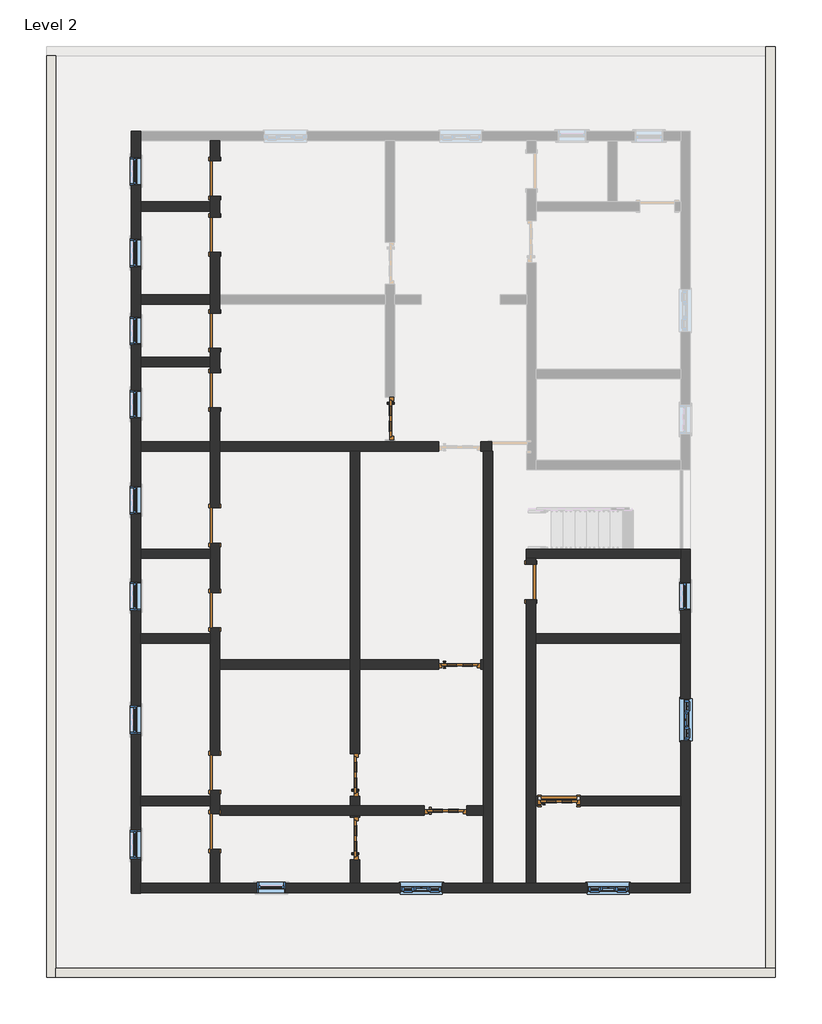
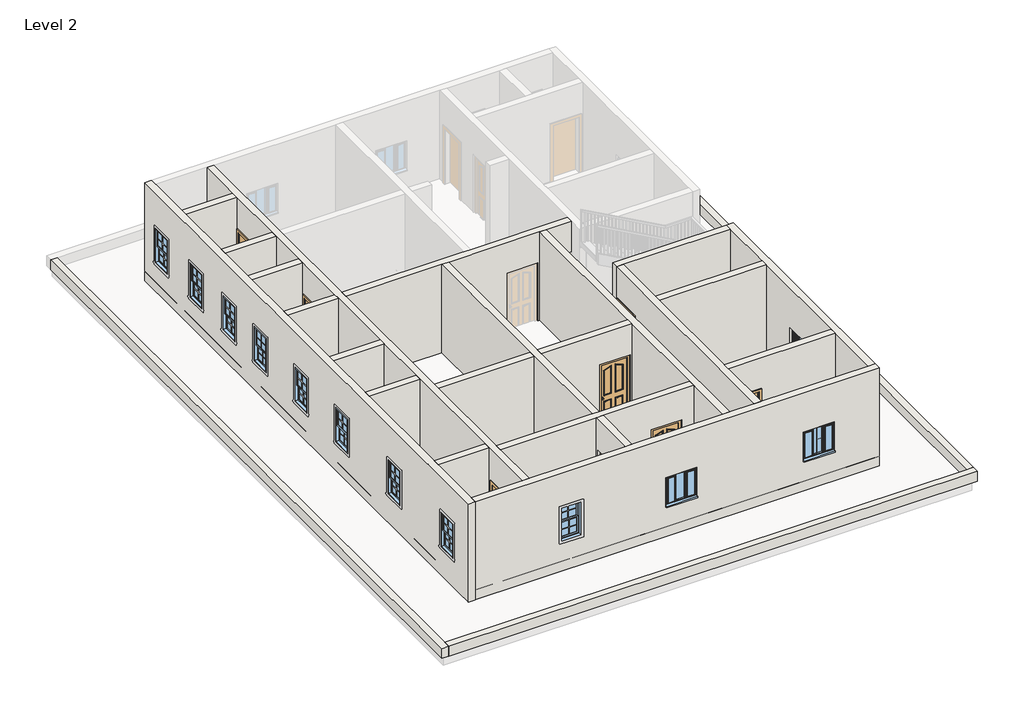
# One storey, part 1 of 3: 22 walls, 16 doors, 13 windows.
"""IFC4 building model written with IfcOpenShell, lengths in millimetres."""

from ifc_helpers import new_model, si_unit, frame, origin, place, context, project, spatial, polyline, outline, extrude, faceted_brep, transform, mapped, element, save
from components import doors_extsgl_12_910x2110mm_9a09825e, doors_extsgl_12_910x2110mm_ece77ece, door_fadea3f2, door_53b1b562, window_679d2811, windows_tpl_w_glazing_cross_bars_910x910mm_4aa0f884

model = new_model("IFC4")

# Units and contexts
model_context = context("Model", 3, world=origin())
ifc_project = project(units=[si_unit("LENGTHUNIT", "METRE", prefix="MILLI")], contexts=[model_context])

# Site, building, storey
site = spatial("IfcSite", under=ifc_project)
building = spatial("IfcBuilding", under=site)
storey = spatial("IfcBuildingStorey", under=building, Name="Level 2", Elevation=3048.0)

# Doors
placement = place(None, origin())
doors_extsgl_12_910x2110mm_shape = doors_extsgl_12_910x2110mm_9a09825e(model_context)
element("IfcDoor", 1, ObjectType="Doors_ExtSgl_12 : 910x2110mm", at=placement, inside=storey, context=model_context, shape_type="MappedRepresentation", body=[
    mapped(doors_extsgl_12_910x2110mm_shape, transform((-4887.6876145, 1213.3404944, 3048.0), x_axis=(0.0, -1.0, 0.0), y_axis=(1.0, 0.0, 0.0), z_axis=(0.0, 0.0, 1.0))),
])
doors_extsgl_12_910x2110mm_2_shape = doors_extsgl_12_910x2110mm_ece77ece(model_context)
element("IfcDoor", 2, ObjectType="Doors_ExtSgl_12 : 910x2110mm", at=placement, inside=storey, context=model_context, shape_type="MappedRepresentation", body=[
    mapped(doors_extsgl_12_910x2110mm_2_shape, transform((-5649.6876145, -6482.8595056, 3048.0), x_axis=(0.0, 1.0, 0.0), y_axis=(-1.0, 0.0, 0.0), z_axis=(0.0, 0.0, 1.0))),
])
element("IfcDoor", 3, ObjectType="Doors_ExtSgl_12 : 910x2110mm", at=placement, inside=storey, context=model_context, shape_type="MappedRepresentation", body=[
    mapped(doors_extsgl_12_910x2110mm_2_shape, transform((-1242.7876145, -7041.6595056, 3048.0), x_axis=(1.0, 0.0, 0.0), y_axis=(0.0, 1.0, 0.0), z_axis=(0.0, 0.0, 1.0))),
])
element("IfcDoor", 4, ObjectType="Doors_ExtSgl_12 : 910x2110mm", at=placement, inside=storey, context=model_context, shape_type="MappedRepresentation", body=[
    mapped(doors_extsgl_12_910x2110mm_2_shape, transform((-5649.6876145, -7854.4595056, 3048.0), x_axis=(0.0, 1.0, 0.0), y_axis=(-1.0, 0.0, 0.0), z_axis=(0.0, 0.0, 1.0))),
])
element("IfcDoor", 5, ObjectType="Doors_ExtSgl_12 : 910x2110mm", at=placement, inside=storey, context=model_context, shape_type="MappedRepresentation", body=[
    mapped(doors_extsgl_12_910x2110mm_2_shape, transform((-3693.8876145, -7244.8595056, 3048.0), x_axis=(1.0, 0.0, 0.0), y_axis=(0.0, 1.0, 0.0), z_axis=(0.0, 0.0, 1.0))),
])
element("IfcDoor", 6, ObjectType="Doors_ExtSgl_12 : 910x2110mm", at=placement, inside=storey, context=model_context, shape_type="MappedRepresentation", body=[
    mapped(doors_extsgl_12_910x2110mm_2_shape, transform((-3389.0876145, -4095.2595056, 3048.0), x_axis=(1.0, 0.0, 0.0), y_axis=(0.0, 1.0, 0.0), z_axis=(0.0, 0.0, 1.0))),
])
door_shape = door_fadea3f2(model_context)
element("IfcDoor", 7, ObjectType="Single-Flush : 30\" x 80\"", at=placement, inside=storey, context=model_context, shape_type="MappedRepresentation", body=[
    mapped(door_shape, transform((-8672.2876145, 5175.7404944, 3048.0), x_axis=(0.0, 1.0, 0.0), y_axis=(-1.0, 0.0, 0.0), z_axis=(0.0, 0.0, 1.0))),
])
element("IfcDoor", 8, ObjectType="Single-Flush : 30\" x 80\"", at=placement, inside=storey, context=model_context, shape_type="MappedRepresentation", body=[
    mapped(door_shape, transform((-8672.2876145, -7702.0595056, 3048.0), x_axis=(0.0, 1.0, 0.0), y_axis=(-1.0, 0.0, 0.0), z_axis=(0.0, 0.0, 1.0))),
])
element("IfcDoor", 9, ObjectType="Single-Flush : 30\" x 80\"", at=placement, inside=storey, context=model_context, shape_type="MappedRepresentation", body=[
    mapped(door_shape, transform((-1852.3876145, -2317.2595056, 3048.0), x_axis=(0.0, -1.0, 0.0), y_axis=(1.0, 0.0, 0.0), z_axis=(0.0, 0.0, 1.0))),
])
element("IfcDoor", 10, ObjectType="Single-Flush : 30\" x 80\"", at=placement, inside=storey, context=model_context, shape_type="MappedRepresentation", body=[
    mapped(door_shape, transform((-1242.7876145, -7041.6595056, 3048.0), x_axis=(1.0, 0.0, 0.0), y_axis=(0.0, 1.0, 0.0), z_axis=(0.0, 0.0, 1.0))),
])
door_2_shape = door_53b1b562(model_context)
element("IfcDoor", 11, ObjectType="Single-Flush : 30\" x 80\"", at=placement, inside=storey, context=model_context, shape_type="MappedRepresentation", body=[
    mapped(door_2_shape, transform((-8672.2876145, 6394.9404944, 3048.0), x_axis=(0.0, -1.0, 0.0), y_axis=(1.0, 0.0, 0.0), z_axis=(0.0, 0.0, 1.0))),
])
element("IfcDoor", 12, ObjectType="Single-Flush : 30\" x 80\"", at=placement, inside=storey, context=model_context, shape_type="MappedRepresentation", body=[
    mapped(door_2_shape, transform((-8672.2876145, 3105.6404944, 3048.0), x_axis=(0.0, -1.0, 0.0), y_axis=(1.0, 0.0, 0.0), z_axis=(0.0, 0.0, 1.0))),
])
element("IfcDoor", 13, ObjectType="Single-Flush : 30\" x 80\"", at=placement, inside=storey, context=model_context, shape_type="MappedRepresentation", body=[
    mapped(door_2_shape, transform((-8672.2876145, 1822.9404944, 3048.0), x_axis=(0.0, -1.0, 0.0), y_axis=(1.0, 0.0, 0.0), z_axis=(0.0, 0.0, 1.0))),
])
element("IfcDoor", 14, ObjectType="Single-Flush : 30\" x 80\"", at=placement, inside=storey, context=model_context, shape_type="MappedRepresentation", body=[
    mapped(door_2_shape, transform((-8672.2876145, -1098.0595056, 3048.0), x_axis=(0.0, -1.0, 0.0), y_axis=(1.0, 0.0, 0.0), z_axis=(0.0, 0.0, 1.0))),
])
element("IfcDoor", 15, ObjectType="Single-Flush : 30\" x 80\"", at=placement, inside=storey, context=model_context, shape_type="MappedRepresentation", body=[
    mapped(door_2_shape, transform((-8672.2876145, -2926.8595056, 3048.0), x_axis=(0.0, -1.0, 0.0), y_axis=(1.0, 0.0, 0.0), z_axis=(0.0, 0.0, 1.0))),
])
element("IfcDoor", 16, ObjectType="Single-Flush : 30\" x 80\"", at=placement, inside=storey, context=model_context, shape_type="MappedRepresentation", body=[
    mapped(door_2_shape, transform((-8672.2876145, -6432.0595056, 3048.0), x_axis=(0.0, -1.0, 0.0), y_axis=(1.0, 0.0, 0.0), z_axis=(0.0, 0.0, 1.0))),
])

# Walls
element("IfcWall", 17, ObjectType="4.5\"", at=placement, inside=storey, context=model_context, shape_type="Brep", body=[
    faceted_brep([(-8773.8876145, -6813.0595056, 3048.0), (-8773.8876145, -6940.0595056, 3048.0), (-8773.8876145, -7143.2595056, 3048.0), (-8773.8876145, -7321.0595056, 3048.0), (-8773.8876145, -7321.0595056, 5080.0), (-8773.8876145, -8083.0595056, 5080.0), (-8773.8876145, -8083.0595056, 3048.0), (-8773.8876145, -8819.6595056, 3048.0), (-8773.8876145, -8819.6595056, 6096.0), (-8773.8876145, -7143.2595056, 6096.0), (-8773.8876145, -6940.0595056, 6096.0), (-8773.8876145, -3638.0595056, 6096.0), (-8773.8876145, -3434.8595056, 6096.0), (-8773.8876145, -1809.2595056, 6096.0), (-8773.8876145, -1606.0595056, 6096.0), (-8773.8876145, 502.1404944, 6096.0), (-8773.8876145, 705.3404944, 6096.0), (-8773.8876145, 2330.9404944, 6096.0), (-8773.8876145, 2534.1404944, 6096.0), (-8773.8876145, 3677.1404944, 6096.0), (-8773.8876145, 3880.3404944, 6096.0), (-8773.8876145, 5683.7404944, 6096.0), (-8773.8876145, 5886.9404944, 6096.0), (-8773.8876145, 7207.7404944, 6096.0), (-8773.8876145, 7207.7404944, 3048.0), (-8773.8876145, 6775.9404944, 3048.0), (-8773.8876145, 6775.9404944, 5080.0), (-8773.8876145, 6013.9404944, 5080.0), (-8773.8876145, 6013.9404944, 3048.0), (-8773.8876145, 5886.9404944, 3048.0), (-8773.8876145, 5683.7404944, 3048.0), (-8773.8876145, 5556.7404944, 3048.0), (-8773.8876145, 5556.7404944, 5080.0), (-8773.8876145, 4794.7404944, 5080.0), (-8773.8876145, 4794.7404944, 3048.0), (-8773.8876145, 3880.3404944, 3048.0), (-8773.8876145, 3677.1404944, 3048.0), (-8773.8876145, 3486.6404944, 3048.0), (-8773.8876145, 3486.6404944, 5080.0), (-8773.8876145, 2724.6404944, 5080.0), (-8773.8876145, 2724.6404944, 3048.0), (-8773.8876145, 2534.1404944, 3048.0), (-8773.8876145, 2330.9404944, 3048.0), (-8773.8876145, 2203.9404944, 3048.0), (-8773.8876145, 2203.9404944, 5080.0), (-8773.8876145, 1441.9404944, 5080.0), (-8773.8876145, 1441.9404944, 3048.0), (-8773.8876145, 705.3404944, 3048.0), (-8773.8876145, 502.1404944, 3048.0), (-8773.8876145, -717.0595056, 3048.0), (-8773.8876145, -717.0595056, 5080.0), (-8773.8876145, -1479.0595056, 5080.0), (-8773.8876145, -1479.0595056, 3048.0), (-8773.8876145, -1606.0595056, 3048.0), (-8773.8876145, -1809.2595056, 3048.0), (-8773.8876145, -2545.8595056, 3048.0), (-8773.8876145, -2545.8595056, 5080.0), (-8773.8876145, -3307.8595056, 5080.0), (-8773.8876145, -3307.8595056, 3048.0), (-8773.8876145, -3434.8595056, 3048.0), (-8773.8876145, -3638.0595056, 3048.0), (-8773.8876145, -6051.0595056, 3048.0), (-8773.8876145, -6051.0595056, 5080.0), (-8773.8876145, -6813.0595056, 5080.0), (-8570.6876145, -7321.0595056, 5080.0), (-8570.6876145, -7321.0595056, 3048.0), (-8570.6876145, -7143.2595056, 3048.0), (-8570.6876145, -6813.0595056, 3048.0), (-8570.6876145, -6813.0595056, 5080.0), (-8570.6876145, -6051.0595056, 5080.0), (-8570.6876145, -6051.0595056, 3048.0), (-8570.6876145, -4196.8595056, 3048.0), (-8570.6876145, -3993.6595056, 3048.0), (-8570.6876145, -3307.8595056, 3048.0), (-8570.6876145, -3307.8595056, 5080.0), (-8570.6876145, -2545.8595056, 5080.0), (-8570.6876145, -2545.8595056, 3048.0), (-8570.6876145, -1479.0595056, 3048.0), (-8570.6876145, -1479.0595056, 5080.0), (-8570.6876145, -717.0595056, 5080.0), (-8570.6876145, -717.0595056, 3048.0), (-8570.6876145, 502.1404944, 3048.0), (-8570.6876145, 705.3404944, 3048.0), (-8570.6876145, 1441.9404944, 3048.0), (-8570.6876145, 1441.9404944, 5080.0), (-8570.6876145, 2203.9404944, 5080.0), (-8570.6876145, 2203.9404944, 3048.0), (-8570.6876145, 2724.6404944, 3048.0), (-8570.6876145, 2724.6404944, 5080.0), (-8570.6876145, 3486.6404944, 5080.0), (-8570.6876145, 3486.6404944, 3048.0), (-8570.6876145, 3677.1404944, 3048.0), (-8570.6876145, 3880.3404944, 3048.0), (-8570.6876145, 4794.7404944, 3048.0), (-8570.6876145, 4794.7404944, 5080.0), (-8570.6876145, 5556.7404944, 5080.0), (-8570.6876145, 5556.7404944, 3048.0), (-8570.6876145, 6013.9404944, 3048.0), (-8570.6876145, 6013.9404944, 5080.0), (-8570.6876145, 6775.9404944, 5080.0), (-8570.6876145, 6775.9404944, 3048.0), (-8570.6876145, 7207.7404944, 3048.0), (-8570.6876145, 7207.7404944, 6096.0), (-8570.6876145, 3880.3404944, 6096.0), (-8570.6876145, 3677.1404944, 6096.0), (-8570.6876145, 705.3404944, 6096.0), (-8570.6876145, 502.1404944, 6096.0), (-8570.6876145, -3993.6595056, 6096.0), (-8570.6876145, -4196.8595056, 6096.0), (-8570.6876145, -7143.2595056, 6096.0), (-8570.6876145, -7346.4595056, 6096.0), (-8570.6876145, -8819.6595056, 6096.0), (-8570.6876145, -8819.6595056, 3048.0), (-8570.6876145, -8083.0595056, 3048.0), (-8570.6876145, -8083.0595056, 5080.0)], [[[0, 1, 2, 3, 4, 5, 6, 7, 8, 9, 10, 11, 12, 13, 14, 15, 16, 17, 18, 19, 20, 21, 22, 23, 24, 25, 26, 27, 28, 29, 30, 31, 32, 33, 34, 35, 36, 37, 38, 39, 40, 41, 42, 43, 44, 45, 46, 47, 48, 49, 50, 51, 52, 53, 54, 55, 56, 57, 58, 59, 60, 61, 62, 63]], [[64, 65, 66, 67, 68, 69, 70, 71, 72, 73, 74, 75, 76, 77, 78, 79, 80, 81, 82, 83, 84, 85, 86, 87, 88, 89, 90, 91, 92, 93, 94, 95, 96, 97, 98, 99, 100, 101, 102, 103, 104, 105, 106, 107, 108, 109, 110, 111, 112, 113, 114]], [[25, 24, 101, 100]], [[97, 96, 31, 30, 29, 28]], [[37, 36, 35, 34, 93, 92, 91, 90]], [[43, 42, 41, 40, 87, 86]], [[49, 48, 47, 46, 83, 82, 81, 80]], [[55, 54, 53, 52, 77, 76]], [[61, 60, 59, 58, 73, 72, 71, 70]], [[113, 112, 7, 6]], [[67, 66, 65, 3, 2, 1, 0]], [[23, 22, 21, 20, 19, 18, 17, 16, 15, 14, 13, 12, 11, 10, 9, 8, 111, 110, 109, 108, 107, 106, 105, 104, 103, 102]], [[8, 7, 112, 111]], [[24, 23, 102, 101]], [[98, 97, 28, 27]], [[99, 98, 27, 26]], [[100, 99, 26, 25]], [[32, 31, 96, 95]], [[33, 32, 95, 94]], [[34, 33, 94, 93]], [[88, 87, 40, 39]], [[89, 88, 39, 38]], [[90, 89, 38, 37]], [[84, 83, 46, 45]], [[85, 84, 45, 44]], [[86, 85, 44, 43]], [[78, 77, 52, 51]], [[79, 78, 51, 50]], [[80, 79, 50, 49]], [[74, 73, 58, 57]], [[75, 74, 57, 56]], [[76, 75, 56, 55]], [[68, 67, 0, 63]], [[69, 68, 63, 62]], [[70, 69, 62, 61]], [[4, 3, 65, 64]], [[5, 4, 64, 114]], [[6, 5, 114, 113]]]),
])
element("IfcWall", 18, ObjectType="4.5\"", at=placement, inside=storey, context=model_context, shape_type="SweptSolid", body=[
    extrude(outline(polyline([(-8773.8876145, 5683.7404944), (-10272.4876145, 5683.7404944), (-10272.4876145, 5886.9404944), (-8773.8876145, 5886.9404944), (-8773.8876145, 5683.7404944)])), frame((0.0, 0.0, 3048.0), z_axis=(0.0, 0.0, 1.0), x_axis=(1.0, 0.0, 0.0)), (0.0, 0.0, 1.0), 3048.0),
])
element("IfcWall", 19, ObjectType="4.5\"", at=placement, inside=storey, context=model_context, shape_type="SweptSolid", body=[
    extrude(outline(polyline([(-8773.8876145, 3677.1404944), (-10272.4876145, 3677.1404944), (-10272.4876145, 3880.3404944), (-8773.8876145, 3880.3404944), (-8773.8876145, 3677.1404944)])), frame((0.0, 0.0, 3048.0), z_axis=(0.0, 0.0, 1.0), x_axis=(1.0, 0.0, 0.0)), (0.0, 0.0, 1.0), 3048.0),
])
element("IfcWall", 20, ObjectType="4.5\"", at=placement, inside=storey, context=model_context, shape_type="SweptSolid", body=[
    extrude(outline(polyline([(-8773.8876145, 2330.9404944), (-10272.4876145, 2330.9404944), (-10272.4876145, 2534.1404944), (-8773.8876145, 2534.1404944), (-8773.8876145, 2330.9404944)])), frame((0.0, 0.0, 3048.0), z_axis=(0.0, 0.0, 1.0), x_axis=(1.0, 0.0, 0.0)), (0.0, 0.0, 1.0), 3048.0),
])
element("IfcWall", 21, ObjectType="4.5\"", at=placement, inside=storey, context=model_context, shape_type="Brep", body=[
    faceted_brep([(-10272.4876145, 502.1404944, 6096.0), (-10272.4876145, 502.1404944, 3048.0), (-8773.8876145, 502.1404944, 3048.0), (-8773.8876145, 502.1404944, 6096.0), (-10272.4876145, 705.3404944, 3048.0), (-10272.4876145, 705.3404944, 6096.0), (-8773.8876145, 705.3404944, 6096.0), (-8773.8876145, 705.3404944, 3048.0)], [[[0, 1, 2, 3]], [[4, 5, 6, 7]], [[1, 4, 7, 2]], [[5, 0, 3, 6]], [[1, 0, 5, 4]], [[3, 2, 7, 6]]]),
    faceted_brep([(-1941.2876145, 502.1404944, 5080.0), (-1941.2876145, 502.1404944, 6096.0), (-2677.8876145, 502.1404944, 6096.0), (-2881.0876145, 502.1404944, 6096.0), (-5548.0876145, 502.1404944, 6096.0), (-5751.2876145, 502.1404944, 6096.0), (-8570.6876145, 502.1404944, 6096.0), (-8570.6876145, 502.1404944, 3048.0), (-5751.2876145, 502.1404944, 3048.0), (-5548.0876145, 502.1404944, 3048.0), (-3844.0876145, 502.1404944, 3048.0), (-3844.0876145, 502.1404944, 5158.0), (-2934.0876145, 502.1404944, 5158.0), (-2934.0876145, 502.1404944, 3048.0), (-2881.0876145, 502.1404944, 3048.0), (-2690.5876145, 502.1404944, 3048.0), (-2690.5876145, 502.1404944, 5080.0), (-1941.2876145, 705.3404944, 6096.0), (-1941.2876145, 705.3404944, 5080.0), (-2690.5876145, 705.3404944, 5080.0), (-2690.5876145, 705.3404944, 3048.0), (-2934.0876145, 705.3404944, 3048.0), (-2934.0876145, 705.3404944, 5158.0), (-3844.0876145, 705.3404944, 5158.0), (-3844.0876145, 705.3404944, 3048.0), (-4786.0876145, 705.3404944, 3048.0), (-4989.2876145, 705.3404944, 3048.0), (-8570.6876145, 705.3404944, 3048.0), (-8570.6876145, 705.3404944, 6096.0), (-4989.2876145, 705.3404944, 6096.0), (-4786.0876145, 705.3404944, 6096.0)], [[[0, 1, 2, 3, 4, 5, 6, 7, 8, 9, 10, 11, 12, 13, 14, 15, 16]], [[17, 18, 19, 20, 21, 22, 23, 24, 25, 26, 27, 28, 29, 30]], [[20, 15, 14, 13, 21]], [[24, 10, 9, 8, 7, 27, 26, 25]], [[1, 17, 30, 29, 28, 6, 5, 4, 3, 2]], [[7, 6, 28, 27]], [[17, 1, 0, 18]], [[16, 19, 18, 0]], [[19, 16, 15, 20]], [[24, 23, 11, 10]], [[22, 21, 13, 12]], [[23, 22, 12, 11]]]),
])
element("IfcWall", 22, ObjectType="4.5\"", at=placement, inside=storey, context=model_context, shape_type="SweptSolid", body=[
    extrude(outline(polyline([(-8773.8876145, -1809.2595056), (-10272.4876145, -1809.2595056), (-10272.4876145, -1606.0595056), (-8773.8876145, -1606.0595056), (-8773.8876145, -1809.2595056)])), frame((0.0, 0.0, 3048.0), z_axis=(0.0, 0.0, 1.0), x_axis=(1.0, 0.0, 0.0)), (0.0, 0.0, 1.0), 3048.0),
])
element("IfcWall", 23, ObjectType="4.5\"", at=placement, inside=storey, context=model_context, shape_type="SweptSolid", body=[
    extrude(outline(polyline([(-8773.8876145, -3638.0595056), (-10272.4876145, -3638.0595056), (-10272.4876145, -3434.8595056), (-8773.8876145, -3434.8595056), (-8773.8876145, -3638.0595056)])), frame((0.0, 0.0, 3048.0), z_axis=(0.0, 0.0, 1.0), x_axis=(1.0, 0.0, 0.0)), (0.0, 0.0, 1.0), 3048.0),
])
element("IfcWall", 24, ObjectType="4.5\"", at=placement, inside=storey, context=model_context, shape_type="SweptSolid", body=[
    extrude(outline(polyline([(-8773.8876145, -7143.2595056), (-10272.4876145, -7143.2595056), (-10272.4876145, -6940.0595056), (-8773.8876145, -6940.0595056), (-8773.8876145, -7143.2595056)])), frame((0.0, 0.0, 3048.0), z_axis=(0.0, 0.0, 1.0), x_axis=(1.0, 0.0, 0.0)), (0.0, 0.0, 1.0), 3048.0),
])
element("IfcWall", 25, ObjectType="4.5\"", at=placement, inside=storey, context=model_context, shape_type="Brep", body=[
    faceted_brep([(-3238.8876145, -7346.4595056, 5158.0), (-3238.8876145, -7346.4595056, 3048.0), (-2881.0876145, -7346.4595056, 3048.0), (-2881.0876145, -7346.4595056, 6096.0), (-5548.0876145, -7346.4595056, 6096.0), (-5751.2876145, -7346.4595056, 6096.0), (-8570.6876145, -7346.4595056, 6096.0), (-8570.6876145, -7346.4595056, 3048.0), (-5751.2876145, -7346.4595056, 3048.0), (-5548.0876145, -7346.4595056, 3048.0), (-4148.8876145, -7346.4595056, 3048.0), (-4148.8876145, -7346.4595056, 5158.0), (-2881.0876145, -7143.2595056, 3048.0), (-3238.8876145, -7143.2595056, 3048.0), (-3238.8876145, -7143.2595056, 5158.0), (-4148.8876145, -7143.2595056, 5158.0), (-4148.8876145, -7143.2595056, 3048.0), (-5548.0876145, -7143.2595056, 3048.0), (-5751.2876145, -7143.2595056, 3048.0), (-8570.6876145, -7143.2595056, 3048.0), (-8570.6876145, -7143.2595056, 6096.0), (-5751.2876145, -7143.2595056, 6096.0), (-5548.0876145, -7143.2595056, 6096.0), (-2881.0876145, -7143.2595056, 6096.0), (-8570.6876145, -7321.0595056, 3048.0)], [[[0, 1, 2, 3, 4, 5, 6, 7, 8, 9, 10, 11]], [[12, 13, 14, 15, 16, 17, 18, 19, 20, 21, 22, 23]], [[2, 1, 13, 12]], [[10, 9, 8, 7, 24, 19, 18, 17, 16]], [[6, 5, 4, 3, 23, 22, 21, 20]], [[7, 6, 20, 19, 24]], [[3, 2, 12, 23]], [[16, 15, 11, 10]], [[14, 13, 1, 0]], [[15, 14, 0, 11]]]),
])
element("IfcWall", 26, ObjectType="4.5\"", at=placement, inside=storey, context=model_context, shape_type="Brep", body=[
    faceted_brep([(-5751.2876145, -8819.6595056, 3048.0), (-5751.2876145, -8819.6595056, 6096.0), (-5751.2876145, -7346.4595056, 6096.0), (-5751.2876145, -7346.4595056, 3048.0), (-5751.2876145, -7399.4595056, 3048.0), (-5751.2876145, -7399.4595056, 5158.0), (-5751.2876145, -8309.4595056, 5158.0), (-5751.2876145, -8309.4595056, 3048.0), (-5548.0876145, -8819.6595056, 6096.0), (-5548.0876145, -8819.6595056, 3048.0), (-5548.0876145, -8309.4595056, 3048.0), (-5548.0876145, -8309.4595056, 5158.0), (-5548.0876145, -7399.4595056, 5158.0), (-5548.0876145, -7399.4595056, 3048.0), (-5548.0876145, -7346.4595056, 3048.0), (-5548.0876145, -7346.4595056, 6096.0)], [[[0, 1, 2, 3, 4, 5, 6, 7]], [[8, 9, 10, 11, 12, 13, 14, 15]], [[9, 0, 7, 10]], [[13, 4, 3, 14]], [[1, 8, 15, 2]], [[1, 0, 9, 8]], [[3, 2, 15, 14]], [[7, 6, 11, 10]], [[5, 4, 13, 12]], [[6, 5, 12, 11]]]),
    faceted_brep([(-5751.2876145, 502.1404944, 6096.0), (-5751.2876145, 502.1404944, 3048.0), (-5751.2876145, -3993.6595056, 3048.0), (-5751.2876145, -4196.8595056, 3048.0), (-5751.2876145, -6027.8595056, 3048.0), (-5751.2876145, -6027.8595056, 5158.0), (-5751.2876145, -6937.8595056, 5158.0), (-5751.2876145, -6937.8595056, 3048.0), (-5751.2876145, -7143.2595056, 3048.0), (-5751.2876145, -7143.2595056, 6096.0), (-5751.2876145, -4196.8595056, 6096.0), (-5751.2876145, -3993.6595056, 6096.0), (-5548.0876145, 502.1404944, 3048.0), (-5548.0876145, 502.1404944, 6096.0), (-5548.0876145, -3993.6595056, 6096.0), (-5548.0876145, -4196.8595056, 6096.0), (-5548.0876145, -7143.2595056, 6096.0), (-5548.0876145, -7143.2595056, 3048.0), (-5548.0876145, -6937.8595056, 3048.0), (-5548.0876145, -6937.8595056, 5158.0), (-5548.0876145, -6027.8595056, 5158.0), (-5548.0876145, -6027.8595056, 3048.0), (-5548.0876145, -4196.8595056, 3048.0), (-5548.0876145, -3993.6595056, 3048.0)], [[[0, 1, 2, 3, 4, 5, 6, 7, 8, 9, 10, 11]], [[12, 13, 14, 15, 16, 17, 18, 19, 20, 21, 22, 23]], [[1, 12, 23, 22, 21, 4, 3, 2]], [[7, 18, 17, 8]], [[13, 0, 11, 10, 9, 16, 15, 14]], [[1, 0, 13, 12]], [[9, 8, 17, 16]], [[7, 6, 19, 18]], [[5, 4, 21, 20]], [[6, 5, 20, 19]]]),
])
element("IfcWall", 27, ObjectType="4.5\"", at=placement, inside=storey, context=model_context, shape_type="SweptSolid", body=[
    extrude(outline(polyline([(-8570.6876145, -4196.8595056), (-8570.6876145, -3993.6595056), (-5751.2876145, -3993.6595056), (-5751.2876145, -4196.8595056), (-8570.6876145, -4196.8595056)])), frame((0.0, 0.0, 3048.0), z_axis=(0.0, 0.0, 1.0), x_axis=(1.0, 0.0, 0.0)), (0.0, 0.0, 1.0), 3048.0),
    extrude(outline(polyline([(3048.0, -2881.0876145), (6096.0, -2881.0876145), (6096.0, -5548.0876145), (3048.0, -5548.0876145), (3048.0, -3844.0876145), (5158.0, -3844.0876145), (5158.0, -2934.0876145), (3048.0, -2934.0876145), (3048.0, -2881.0876145)])), frame((0.0, -4196.8595056, 0.0), z_axis=(0.0, 1.0, 0.0), x_axis=(0.0, 0.0, 1.0)), (0.0, 0.0, 1.0), 203.2),
])
element("IfcWall", 28, ObjectType="4.5\"", at=placement, inside=storey, context=model_context, shape_type="Brep", body=[
    faceted_brep([(-2881.0876145, 502.1404944, 3048.0), (-2881.0876145, -3993.6595056, 3048.0), (-2881.0876145, -4196.8595056, 3048.0), (-2881.0876145, -7143.2595056, 3048.0), (-2881.0876145, -7346.4595056, 3048.0), (-2881.0876145, -8819.6595056, 3048.0), (-2881.0876145, -8819.6595056, 6096.0), (-2881.0876145, -7346.4595056, 6096.0), (-2881.0876145, -7143.2595056, 6096.0), (-2881.0876145, -4196.8595056, 6096.0), (-2881.0876145, -3993.6595056, 6096.0), (-2881.0876145, 502.1404944, 6096.0), (-2677.8876145, 502.1404944, 3048.0), (-2677.8876145, 502.1404944, 6096.0), (-2677.8876145, -8819.6595056, 6096.0), (-2677.8876145, -8819.6595056, 3048.0), (-2690.5876145, 502.1404944, 3048.0)], [[[0, 1, 2, 3, 4, 5, 6, 7, 8, 9, 10, 11]], [[12, 13, 14, 15]], [[5, 4, 3, 2, 1, 0, 16, 12, 15]], [[11, 10, 9, 8, 7, 6, 14, 13]], [[6, 5, 15, 14]], [[0, 11, 13, 12, 16]]]),
])
element("IfcWall", 29, ObjectType="4.5\"", at=placement, inside=storey, context=model_context, shape_type="Brep", body=[
    faceted_brep([(1386.1123855, -1606.0595056, 3048.0), (-1953.9876145, -1606.0595056, 3048.0), (-1953.9876145, -1606.0595056, 6096.0), (1386.1123855, -1606.0595056, 6096.0), (1386.1123855, -1809.2595056, 3048.0), (1386.1123855, -1809.2595056, 6096.0), (-1750.7876145, -1809.2595056, 6096.0), (-1953.9876145, -1809.2595056, 6096.0), (-1953.9876145, -1809.2595056, 3048.0), (-1750.7876145, -1809.2595056, 3048.0)], [[[0, 1, 2, 3]], [[4, 5, 6, 7, 8, 9]], [[1, 0, 4, 9, 8]], [[3, 2, 7, 6, 5]], [[0, 3, 5, 4]], [[2, 1, 8, 7]]]),
])
element("IfcWall", 30, ObjectType="4.5\"", at=placement, inside=storey, context=model_context, shape_type="Brep", body=[
    faceted_brep([(-1953.9876145, -2698.2595056, 5080.0), (-1953.9876145, -2698.2595056, 3048.0), (-1953.9876145, -8819.6595056, 3048.0), (-1953.9876145, -8819.6595056, 6096.0), (-1953.9876145, -1809.2595056, 6096.0), (-1953.9876145, -1809.2595056, 3048.0), (-1953.9876145, -1936.2595056, 3048.0), (-1953.9876145, -1936.2595056, 5080.0), (-1750.7876145, -8819.6595056, 3048.0), (-1750.7876145, -7143.2595056, 3048.0), (-1750.7876145, -6940.0595056, 3048.0), (-1750.7876145, -3638.0595056, 3048.0), (-1750.7876145, -3434.8595056, 3048.0), (-1750.7876145, -2698.2595056, 3048.0), (-1750.7876145, -2698.2595056, 5080.0), (-1750.7876145, -1936.2595056, 5080.0), (-1750.7876145, -1936.2595056, 3048.0), (-1750.7876145, -1809.2595056, 3048.0), (-1750.7876145, -1809.2595056, 6096.0), (-1750.7876145, -3434.8595056, 6096.0), (-1750.7876145, -3638.0595056, 6096.0), (-1750.7876145, -6940.0595056, 6096.0), (-1750.7876145, -7143.2595056, 6096.0), (-1750.7876145, -8819.6595056, 6096.0)], [[[0, 1, 2, 3, 4, 5, 6, 7]], [[8, 9, 10, 11, 12, 13, 14, 15, 16, 17, 18, 19, 20, 21, 22, 23]], [[6, 5, 17, 16]], [[2, 1, 13, 12, 11, 10, 9, 8]], [[4, 3, 23, 22, 21, 20, 19, 18]], [[5, 4, 18, 17]], [[3, 2, 8, 23]], [[14, 13, 1, 0]], [[15, 14, 0, 7]], [[16, 15, 7, 6]]]),
])
element("IfcWall", 31, ObjectType="4.5\"", at=placement, inside=storey, context=model_context, shape_type="SweptSolid", body=[
    extrude(outline(polyline([(6096.0, 1386.1123855), (6096.0, -1750.7876145), (3048.0, -1750.7876145), (3048.0, -1697.7876145), (5158.0, -1697.7876145), (5158.0, -787.7876145), (3048.0, -787.7876145), (3048.0, 1386.1123855), (6096.0, 1386.1123855)])), frame((0.0, -7143.2595056, 0.0), z_axis=(0.0, 1.0, 0.0), x_axis=(0.0, 0.0, 1.0)), (0.0, 0.0, 1.0), 203.2),
])
element("IfcWall", 32, ObjectType="4.5\"", at=placement, inside=storey, context=model_context, shape_type="SweptSolid", body=[
    extrude(outline(polyline([(1386.1123855, -3638.0595056), (-1750.7876145, -3638.0595056), (-1750.7876145, -3434.8595056), (1386.1123855, -3434.8595056), (1386.1123855, -3638.0595056)])), frame((0.0, 0.0, 3048.0), z_axis=(0.0, 0.0, 1.0), x_axis=(1.0, 0.0, 0.0)), (0.0, 0.0, 1.0), 3048.0),
])
element("IfcWall", 33, ObjectType="4.5\"", at=placement, inside=storey, context=model_context, shape_type="Brep", body=[
    faceted_brep([(-12101.2876145, -10851.6595056, 3048.0), (-12101.2876145, -10648.4595056, 3048.0), (-12101.2876145, 9036.5404944, 3048.0), (-12101.2876145, 9036.5404944, 3352.8), (-12101.2876145, -10648.4595056, 3352.8), (-12101.2876145, -10851.6595056, 3352.8), (-12304.4876145, -10851.6595056, 3048.0), (-12304.4876145, -10851.6595056, 3352.8), (-12304.4876145, 9036.5404944, 3352.8), (-12304.4876145, 9036.5404944, 3048.0)], [[[0, 1, 2, 3, 4, 5]], [[6, 7, 8, 9]], [[2, 1, 0, 6, 9]], [[5, 4, 3, 8, 7]], [[0, 5, 7, 6]], [[3, 2, 9, 8]]]),
])
element("IfcWall", 34, ObjectType="4.5\"", at=placement, inside=storey, context=model_context, shape_type="Brep", body=[
    faceted_brep([(3418.1123855, -10648.4595056, 3048.0), (3214.9123855, -10648.4595056, 3048.0), (-12101.2876145, -10648.4595056, 3048.0), (-12101.2876145, -10648.4595056, 3352.8), (3214.9123855, -10648.4595056, 3352.8), (3418.1123855, -10648.4595056, 3352.8), (3418.1123855, -10851.6595056, 3048.0), (3418.1123855, -10851.6595056, 3352.8), (-12101.2876145, -10851.6595056, 3352.8), (-12101.2876145, -10851.6595056, 3048.0)], [[[0, 1, 2, 3, 4, 5]], [[6, 7, 8, 9]], [[2, 1, 0, 6, 9]], [[5, 4, 3, 8, 7]], [[0, 5, 7, 6]], [[3, 2, 9, 8]]]),
])
element("IfcWall", 35, ObjectType="4.5\"", at=placement, inside=storey, context=model_context, shape_type="Brep", body=[
    faceted_brep([(3214.9123855, 9239.7404944, 3048.0), (3214.9123855, 9036.5404944, 3048.0), (3214.9123855, -10648.4595056, 3048.0), (3214.9123855, -10648.4595056, 3352.8), (3214.9123855, 9036.5404944, 3352.8), (3214.9123855, 9239.7404944, 3352.8), (3418.1123855, 9239.7404944, 3048.0), (3418.1123855, 9239.7404944, 3352.8), (3418.1123855, -10648.4595056, 3352.8), (3418.1123855, -10648.4595056, 3048.0)], [[[0, 1, 2, 3, 4, 5]], [[6, 7, 8, 9]], [[2, 1, 0, 6, 9]], [[5, 4, 3, 8, 7]], [[0, 5, 7, 6]], [[3, 2, 9, 8]]]),
])
element("IfcWall", 36, ObjectType="Generic - 9\"", at=placement, inside=storey, context=model_context, shape_type="Brep", body=[
    faceted_brep([(-10475.6876145, 7410.9404944, 3048.0), (-10475.6876145, -9035.5595056, 3048.0), (-10475.6876145, -9035.5595056, 6096.0), (-10475.6876145, 7410.9404944, 6096.0), (-10475.6876145, 6242.5404944, 5029.2), (-10475.6876145, 6242.5404944, 3962.4), (-10475.6876145, 6852.1404944, 3962.4), (-10475.6876145, 6852.1404944, 5029.2), (-10475.6876145, 4477.2404944, 5029.2), (-10475.6876145, 4477.2404944, 3962.4), (-10475.6876145, 5086.8404944, 3962.4), (-10475.6876145, 5086.8404944, 5029.2), (-10475.6876145, 2800.8404944, 5029.2), (-10475.6876145, 2800.8404944, 3962.4), (-10475.6876145, 3410.4404944, 3962.4), (-10475.6876145, 3410.4404944, 5029.2), (-10475.6876145, 1213.3404944, 5029.2), (-10475.6876145, 1213.3404944, 3962.4), (-10475.6876145, 1822.9404944, 3962.4), (-10475.6876145, 1822.9404944, 5029.2), (-10475.6876145, -856.7595056, 5029.2), (-10475.6876145, -856.7595056, 3962.4), (-10475.6876145, -247.1595056, 3962.4), (-10475.6876145, -247.1595056, 5029.2), (-10475.6876145, -2926.8595056, 5029.2), (-10475.6876145, -2926.8595056, 3962.4), (-10475.6876145, -2317.2595056, 3962.4), (-10475.6876145, -2317.2595056, 5029.2), (-10475.6876145, -5593.8595056, 5029.2), (-10475.6876145, -5593.8595056, 3962.4), (-10475.6876145, -4984.2595056, 3962.4), (-10475.6876145, -4984.2595056, 5029.2), (-10475.6876145, -8286.2595056, 5029.2), (-10475.6876145, -8286.2595056, 3962.4), (-10475.6876145, -7676.6595056, 3962.4), (-10475.6876145, -7676.6595056, 5029.2), (-10272.4876145, 7410.9404944, 3048.0), (-10272.4876145, 7410.9404944, 6096.0), (-10272.4876145, 7207.7404944, 6096.0), (-10272.4876145, 5886.9404944, 6096.0), (-10272.4876145, 5683.7404944, 6096.0), (-10272.4876145, 3880.3404944, 6096.0), (-10272.4876145, 3677.1404944, 6096.0), (-10272.4876145, 2534.1404944, 6096.0), (-10272.4876145, 2330.9404944, 6096.0), (-10272.4876145, 705.3404944, 6096.0), (-10272.4876145, 502.1404944, 6096.0), (-10272.4876145, -1606.0595056, 6096.0), (-10272.4876145, -1809.2595056, 6096.0), (-10272.4876145, -3434.8595056, 6096.0), (-10272.4876145, -3638.0595056, 6096.0), (-10272.4876145, -6940.0595056, 6096.0), (-10272.4876145, -7143.2595056, 6096.0), (-10272.4876145, -8819.6595056, 6096.0), (-10272.4876145, -9022.8595056, 6096.0), (-10272.4876145, -9035.5595056, 6096.0), (-10272.4876145, -9035.5595056, 3048.0), (-10272.4876145, -9022.8595056, 3048.0), (-10272.4876145, -8819.6595056, 3048.0), (-10272.4876145, -7143.2595056, 3048.0), (-10272.4876145, -6940.0595056, 3048.0), (-10272.4876145, -3638.0595056, 3048.0), (-10272.4876145, -3434.8595056, 3048.0), (-10272.4876145, -1809.2595056, 3048.0), (-10272.4876145, -1606.0595056, 3048.0), (-10272.4876145, 502.1404944, 3048.0), (-10272.4876145, 705.3404944, 3048.0), (-10272.4876145, 2330.9404944, 3048.0), (-10272.4876145, 2534.1404944, 3048.0), (-10272.4876145, 3677.1404944, 3048.0), (-10272.4876145, 3880.3404944, 3048.0), (-10272.4876145, 5683.7404944, 3048.0), (-10272.4876145, 5886.9404944, 3048.0), (-10272.4876145, 7207.7404944, 3048.0), (-10272.4876145, 6242.5404944, 5029.2), (-10272.4876145, 6852.1404944, 5029.2), (-10272.4876145, 6852.1404944, 3962.4), (-10272.4876145, 6242.5404944, 3962.4), (-10272.4876145, 4477.2404944, 5029.2), (-10272.4876145, 5086.8404944, 5029.2), (-10272.4876145, 5086.8404944, 3962.4), (-10272.4876145, 4477.2404944, 3962.4), (-10272.4876145, 2800.8404944, 5029.2), (-10272.4876145, 3410.4404944, 5029.2), (-10272.4876145, 3410.4404944, 3962.4), (-10272.4876145, 2800.8404944, 3962.4), (-10272.4876145, 1213.3404944, 5029.2), (-10272.4876145, 1822.9404944, 5029.2), (-10272.4876145, 1822.9404944, 3962.4), (-10272.4876145, 1213.3404944, 3962.4), (-10272.4876145, -856.7595056, 5029.2), (-10272.4876145, -247.1595056, 5029.2), (-10272.4876145, -247.1595056, 3962.4), (-10272.4876145, -856.7595056, 3962.4), (-10272.4876145, -2926.8595056, 5029.2), (-10272.4876145, -2317.2595056, 5029.2), (-10272.4876145, -2317.2595056, 3962.4), (-10272.4876145, -2926.8595056, 3962.4), (-10272.4876145, -5593.8595056, 5029.2), (-10272.4876145, -4984.2595056, 5029.2), (-10272.4876145, -4984.2595056, 3962.4), (-10272.4876145, -5593.8595056, 3962.4), (-10272.4876145, -8286.2595056, 5029.2), (-10272.4876145, -7676.6595056, 5029.2), (-10272.4876145, -7676.6595056, 3962.4), (-10272.4876145, -8286.2595056, 3962.4)], [[[0, 1, 2, 3], [4, 5, 6, 7], [8, 9, 10, 11], [12, 13, 14, 15], [16, 17, 18, 19], [20, 21, 22, 23], [24, 25, 26, 27], [28, 29, 30, 31], [32, 33, 34, 35]], [[36, 37, 38, 39, 40, 41, 42, 43, 44, 45, 46, 47, 48, 49, 50, 51, 52, 53, 54, 55, 56, 57, 58, 59, 60, 61, 62, 63, 64, 65, 66, 67, 68, 69, 70, 71, 72, 73], [74, 75, 76, 77], [78, 79, 80, 81], [82, 83, 84, 85], [86, 87, 88, 89], [90, 91, 92, 93], [94, 95, 96, 97], [98, 99, 100, 101], [102, 103, 104, 105]], [[1, 0, 36, 73, 72, 71, 70, 69, 68, 67, 66, 65, 64, 63, 62, 61, 60, 59, 58, 57, 56]], [[2, 1, 56, 55]], [[3, 2, 55, 54, 53, 52, 51, 50, 49, 48, 47, 46, 45, 44, 43, 42, 41, 40, 39, 38, 37]], [[0, 3, 37, 36]], [[5, 4, 74, 77]], [[6, 5, 77, 76]], [[7, 6, 76, 75]], [[4, 7, 75, 74]], [[9, 8, 78, 81]], [[10, 9, 81, 80]], [[11, 10, 80, 79]], [[8, 11, 79, 78]], [[13, 12, 82, 85]], [[14, 13, 85, 84]], [[15, 14, 84, 83]], [[12, 15, 83, 82]], [[17, 16, 86, 89]], [[18, 17, 89, 88]], [[19, 18, 88, 87]], [[16, 19, 87, 86]], [[21, 20, 90, 93]], [[22, 21, 93, 92]], [[23, 22, 92, 91]], [[20, 23, 91, 90]], [[25, 24, 94, 97]], [[26, 25, 97, 96]], [[27, 26, 96, 95]], [[24, 27, 95, 94]], [[29, 28, 98, 101]], [[30, 29, 101, 100]], [[31, 30, 100, 99]], [[28, 31, 99, 98]], [[33, 32, 102, 105]], [[34, 33, 105, 104]], [[35, 34, 104, 103]], [[32, 35, 103, 102]]]),
])
element("IfcWall", 37, ObjectType="Generic - 9\"", at=placement, inside=storey, context=model_context, shape_type="Brep", body=[
    faceted_brep([(-10272.4876145, -9022.8595056, 3048.0), (1589.3123855, -9022.8595056, 3048.0), (1589.3123855, -9022.8595056, 6096.0), (-10272.4876145, -9022.8595056, 6096.0), (-7757.8876145, -9022.8595056, 5029.2), (-7148.2876145, -9022.8595056, 5029.2), (-7148.2876145, -9022.8595056, 3962.4), (-7757.8876145, -9022.8595056, 3962.4), (272.6623855, -9022.8595056, 4872.4), (272.6623855, -9022.8595056, 3962.4), (-637.3376145, -9022.8595056, 3962.4), (-637.3376145, -9022.8595056, 4872.4), (-3759.5876145, -9022.8595056, 4872.4), (-3759.5876145, -9022.8595056, 3962.4), (-4669.5876145, -9022.8595056, 3962.4), (-4669.5876145, -9022.8595056, 4872.4), (-10272.4876145, -8819.6595056, 3048.0), (-10272.4876145, -8819.6595056, 6096.0), (-8773.8876145, -8819.6595056, 6096.0), (-8570.6876145, -8819.6595056, 6096.0), (-5751.2876145, -8819.6595056, 6096.0), (-5548.0876145, -8819.6595056, 6096.0), (-2881.0876145, -8819.6595056, 6096.0), (-2677.8876145, -8819.6595056, 6096.0), (-1953.9876145, -8819.6595056, 6096.0), (-1750.7876145, -8819.6595056, 6096.0), (1386.1123855, -8819.6595056, 6096.0), (1589.3123855, -8819.6595056, 6096.0), (1589.3123855, -8819.6595056, 3048.0), (1386.1123855, -8819.6595056, 3048.0), (-1750.7876145, -8819.6595056, 3048.0), (-1953.9876145, -8819.6595056, 3048.0), (-2677.8876145, -8819.6595056, 3048.0), (-2881.0876145, -8819.6595056, 3048.0), (-5548.0876145, -8819.6595056, 3048.0), (-5751.2876145, -8819.6595056, 3048.0), (-8570.6876145, -8819.6595056, 3048.0), (-8773.8876145, -8819.6595056, 3048.0), (-7757.8876145, -8819.6595056, 5029.2), (-7757.8876145, -8819.6595056, 3962.4), (-7148.2876145, -8819.6595056, 3962.4), (-7148.2876145, -8819.6595056, 5029.2), (272.6623855, -8819.6595056, 4872.4), (-637.3376145, -8819.6595056, 4872.4), (-637.3376145, -8819.6595056, 3962.4), (272.6623855, -8819.6595056, 3962.4), (-3759.5876145, -8819.6595056, 4872.4), (-4669.5876145, -8819.6595056, 4872.4), (-4669.5876145, -8819.6595056, 3962.4), (-3759.5876145, -8819.6595056, 3962.4)], [[[0, 1, 2, 3], [4, 5, 6, 7], [8, 9, 10, 11], [12, 13, 14, 15]], [[16, 17, 18, 19, 20, 21, 22, 23, 24, 25, 26, 27, 28, 29, 30, 31, 32, 33, 34, 35, 36, 37], [38, 39, 40, 41], [42, 43, 44, 45], [46, 47, 48, 49]], [[1, 0, 16, 37, 36, 35, 34, 33, 32, 31, 30, 29, 28]], [[3, 2, 27, 26, 25, 24, 23, 22, 21, 20, 19, 18, 17]], [[0, 3, 17, 16]], [[2, 1, 28, 27]], [[39, 38, 4, 7]], [[40, 39, 7, 6]], [[41, 40, 6, 5]], [[38, 41, 5, 4]], [[9, 8, 42, 45]], [[10, 9, 45, 44]], [[11, 10, 44, 43]], [[8, 11, 43, 42]], [[13, 12, 46, 49]], [[14, 13, 49, 48]], [[15, 14, 48, 47]], [[12, 15, 47, 46]]]),
])
element("IfcWall", 38, ObjectType="Generic - 9\"", at=placement, inside=storey, context=model_context, shape_type="Brep", body=[
    faceted_brep([(1589.3123855, -8819.6595056, 3048.0), (1589.3123855, -1606.0595056, 3048.0), (1589.3123855, -1606.0595056, 6096.0), (1589.3123855, -8819.6595056, 6096.0), (1589.3123855, -4834.0595056, 4872.4), (1589.3123855, -4834.0595056, 3962.4), (1589.3123855, -5744.0595056, 3962.4), (1589.3123855, -5744.0595056, 4872.4), (1589.3123855, -2926.8595056, 5029.2), (1589.3123855, -2317.2595056, 5029.2), (1589.3123855, -2317.2595056, 3962.4), (1589.3123855, -2926.8595056, 3962.4), (1386.1123855, -8819.6595056, 3048.0), (1386.1123855, -8819.6595056, 6096.0), (1386.1123855, -7143.2595056, 6096.0), (1386.1123855, -6940.0595056, 6096.0), (1386.1123855, -3638.0595056, 6096.0), (1386.1123855, -3434.8595056, 6096.0), (1386.1123855, -1809.2595056, 6096.0), (1386.1123855, -1606.0595056, 6096.0), (1386.1123855, -1606.0595056, 3048.0), (1386.1123855, -1809.2595056, 3048.0), (1386.1123855, -3434.8595056, 3048.0), (1386.1123855, -3638.0595056, 3048.0), (1386.1123855, -6940.0595056, 3048.0), (1386.1123855, -7143.2595056, 3048.0), (1386.1123855, -4834.0595056, 4872.4), (1386.1123855, -5744.0595056, 4872.4), (1386.1123855, -5744.0595056, 3962.4), (1386.1123855, -4834.0595056, 3962.4), (1386.1123855, -2926.8595056, 5029.2), (1386.1123855, -2926.8595056, 3962.4), (1386.1123855, -2317.2595056, 3962.4), (1386.1123855, -2317.2595056, 5029.2)], [[[0, 1, 2, 3], [4, 5, 6, 7], [8, 9, 10, 11]], [[12, 13, 14, 15, 16, 17, 18, 19, 20, 21, 22, 23, 24, 25], [26, 27, 28, 29], [30, 31, 32, 33]], [[1, 0, 12, 25, 24, 23, 22, 21, 20]], [[3, 2, 19, 18, 17, 16, 15, 14, 13]], [[0, 3, 13, 12]], [[2, 1, 20, 19]], [[5, 4, 26, 29]], [[6, 5, 29, 28]], [[7, 6, 28, 27]], [[4, 7, 27, 26]], [[31, 30, 8, 11]], [[32, 31, 11, 10]], [[33, 32, 10, 9]], [[30, 33, 9, 8]]]),
])

# Windows
window_shape = window_679d2811(model_context)
element("IfcWindow", 39, ObjectType="Window-Double-Hung : 24\" x 42\"", at=placement, inside=storey, context=model_context, shape_type="MappedRepresentation", body=[
    mapped(window_shape, transform((-10374.0876145, 6547.3404944, 3048.0), x_axis=(0.0, 1.0, 0.0), y_axis=(-1.0, 0.0, 0.0), z_axis=(0.0, 0.0, 1.0))),
])
element("IfcWindow", 40, ObjectType="Window-Double-Hung : 24\" x 42\"", at=placement, inside=storey, context=model_context, shape_type="MappedRepresentation", body=[
    mapped(window_shape, transform((-10374.0876145, 4782.0404944, 3048.0), x_axis=(0.0, 1.0, 0.0), y_axis=(-1.0, 0.0, 0.0), z_axis=(0.0, 0.0, 1.0))),
])
element("IfcWindow", 41, ObjectType="Window-Double-Hung : 24\" x 42\"", at=placement, inside=storey, context=model_context, shape_type="MappedRepresentation", body=[
    mapped(window_shape, transform((-10374.0876145, 3105.6404944, 3048.0), x_axis=(0.0, 1.0, 0.0), y_axis=(-1.0, 0.0, 0.0), z_axis=(0.0, 0.0, 1.0))),
])
element("IfcWindow", 42, ObjectType="Window-Double-Hung : 24\" x 42\"", at=placement, inside=storey, context=model_context, shape_type="MappedRepresentation", body=[
    mapped(window_shape, transform((-10374.0876145, 1518.1404944, 3048.0), x_axis=(0.0, 1.0, 0.0), y_axis=(-1.0, 0.0, 0.0), z_axis=(0.0, 0.0, 1.0))),
])
element("IfcWindow", 43, ObjectType="Window-Double-Hung : 24\" x 42\"", at=placement, inside=storey, context=model_context, shape_type="MappedRepresentation", body=[
    mapped(window_shape, transform((-10374.0876145, -551.9595056, 3048.0), x_axis=(0.0, 1.0, 0.0), y_axis=(-1.0, 0.0, 0.0), z_axis=(0.0, 0.0, 1.0))),
])
element("IfcWindow", 44, ObjectType="Window-Double-Hung : 24\" x 42\"", at=placement, inside=storey, context=model_context, shape_type="MappedRepresentation", body=[
    mapped(window_shape, transform((-10374.0876145, -2622.0595056, 3048.0), x_axis=(0.0, 1.0, 0.0), y_axis=(-1.0, 0.0, 0.0), z_axis=(0.0, 0.0, 1.0))),
])
element("IfcWindow", 45, ObjectType="Window-Double-Hung : 24\" x 42\"", at=placement, inside=storey, context=model_context, shape_type="MappedRepresentation", body=[
    mapped(window_shape, transform((-10374.0876145, -5289.0595056, 3048.0), x_axis=(0.0, 1.0, 0.0), y_axis=(-1.0, 0.0, 0.0), z_axis=(0.0, 0.0, 1.0))),
])
element("IfcWindow", 46, ObjectType="Window-Double-Hung : 24\" x 42\"", at=placement, inside=storey, context=model_context, shape_type="MappedRepresentation", body=[
    mapped(window_shape, transform((-10374.0876145, -7981.4595056, 3048.0), x_axis=(0.0, 1.0, 0.0), y_axis=(-1.0, 0.0, 0.0), z_axis=(0.0, 0.0, 1.0))),
])
element("IfcWindow", 47, ObjectType="Window-Double-Hung : 24\" x 42\"", at=placement, inside=storey, context=model_context, shape_type="MappedRepresentation", body=[
    mapped(window_shape, transform((-7453.0876145, -8921.2595056, 3048.0), x_axis=(1.0, 0.0, 0.0), y_axis=(0.0, 1.0, 0.0), z_axis=(0.0, 0.0, 1.0))),
])
element("IfcWindow", 48, ObjectType="Window-Double-Hung : 24\" x 42\"", at=placement, inside=storey, context=model_context, shape_type="MappedRepresentation", body=[
    mapped(window_shape, transform((1487.7123855, -2622.0595056, 3048.0), x_axis=(0.0, 1.0, 0.0), y_axis=(-1.0, 0.0, 0.0), z_axis=(0.0, 0.0, 1.0))),
])
windows_tpl_w_glazing_cross_bars_910x910mm_shape = windows_tpl_w_glazing_cross_bars_910x910mm_4aa0f884(model_context)
element("IfcWindow", 49, ObjectType="Windows_Tpl_w-Glazing_Cross-Bars : 910x910mm", at=placement, inside=storey, context=model_context, shape_type="MappedRepresentation", body=[
    mapped(windows_tpl_w_glazing_cross_bars_910x910mm_shape, transform((1479.2558177, -5715.7261723, 2762.4), x_axis=(0.0, -1.0, 0.0), y_axis=(1.0, 0.0, 0.0), z_axis=(0.0, 0.0, 1.0))),
])
element("IfcWindow", 50, ObjectType="Windows_Tpl_w-Glazing_Cross-Bars : 910x910mm", at=placement, inside=storey, context=model_context, shape_type="MappedRepresentation", body=[
    mapped(windows_tpl_w_glazing_cross_bars_910x910mm_shape, transform((-609.0042812, -8912.8029378, 2762.4), x_axis=(-1.0, 0.0, 0.0), y_axis=(0.0, -1.0, 0.0), z_axis=(0.0, 0.0, 1.0))),
])
element("IfcWindow", 51, ObjectType="Windows_Tpl_w-Glazing_Cross-Bars : 910x910mm", at=placement, inside=storey, context=model_context, shape_type="MappedRepresentation", body=[
    mapped(windows_tpl_w_glazing_cross_bars_910x910mm_shape, transform((-4641.2542812, -8912.8029378, 2762.4), x_axis=(-1.0, 0.0, 0.0), y_axis=(0.0, -1.0, 0.0), z_axis=(0.0, 0.0, 1.0))),
])

save(model, "model.ifc")

# Revit data of these elements
# Type "Doors_ExtSgl_12 : 910x2110mm"
#   Type Mark = "8"
#   Type Comments = "External Single"
#   Operation = "SingleSwingRight"
#   Construction Type Id = "SGL"
#   Keynote = "L20"
#   Analytic Construction = "Large single-glazed windows"
#   Wrap Layers (Int) from Ext = 0' - 6.98819"
#   Wrap Layers (Ext) from Ext = 0' - 4.03543"
#   Visual Light Transmittance = 0.9
#   Thickness = 0' - 1.73228"
#   Stile Top of Lock rail = 3' - 3.37008"
#   Stile Top Rail = 0' - 5.90551"
#   Stile Shutting = 0' - 4.92126"
#   Stile Muntin Rail = 0' - 4.92126"
#   Stile Lock Rail = 0' - 6.88976"
#   Stile Hanging = 0' - 4.92126"
#   Stile Bottom Rail = 0' - 6.88976"
#   Solar Heat Gain Coefficient = 0.86
#   Rough Width = 2' - 11.82677"
#   Rough Height = 6' - 11.07087"
#   O/A Frame Width = 0' - 2.51969"
#   Heat Transfer Coefficient (U) = 0.979472 BTU/(h·ft²·°F)
#   Handle Z Distance = 3' - 3.37008"
#   Glazing Thickness = 0' - 0.94488"
#   FrameWidth = 0' - 1.65354"
#   FrameOffset - External = 0' - 0.98425"
#   FrameDepth = 0' - 3.50394"
#   Door Panel Width = 2' - 7.77165"
#   Door Panel Thickness = 0' - 1.73228"
#   Door Panel Height = 6' - 6.74016"
#   Cill Thickness = 0' - 2.14567"
#   Cill Projection = 0' - 1.1811"
#   Handle X Distance = 0' - 2.95276"
#   Height = 6' - 11.07087"
#   Structural Tolerance = 0' - 0.25591"
#   Tolerance = 0' - 0.11811"
#   Undercut = 0' - 0.15748"
#   Width = 2' - 11.82677"
#   Cill Extension = 0' - 0.98425"
#   Cavity Closer Width = 0' - 1.9685"
#   Cavity Closer Offset from Ext = 0' - 4.03543"
#   Cavity Closer Depth = 0' - 3.34646"
#   Vis - Ironmongery = yes
#   Vis - Cavity Closers = yes
#   Define Thermal Properties by = 1
#   Function = 1
#   Material Glass = Door - Glazing
#   Material Door = Door - Panel
#   Material Frame = Door - Frame/Mullion
#   Material Ironmongery = Door - Handle
#   Wall Closure = (empty or 0)
# Type "Single-Flush : 30\" x 80\""
#   Type Mark = "5"
#   Construction Type Id = "MDOOR"
#   Assembly Code = "C1020"
#   Analytic Construction = "Metal"
#   Thickness = 0' - 2"
#   Heat Transfer Coefficient (U) = 0.651978 BTU/(h·ft²·°F)
#   Height = 6' - 8"
#   Trim Projection Ext = 0' - 1"
#   Trim Projection Int = 0' - 1"
#   Trim Width = 0' - 3"
#   Width = 2' - 6"
#   Define Thermal Properties by = 1
#   Define Thermal Properties by = 1
#   Door Material = Door - Panel
#   Frame Material = Door - Frame
#   Visual Light Transmittance = 0
#   Solar Heat Gain Coefficient = 0
#   Function = (empty or 0)
#   Wall Closure = (empty or 0)
# Type "4.5\""
#   Assembly Code = "B2010"
#   Layers, outside or top first: 0' - 8" no material (function 1)
# Type "Generic - 9\""
#   Assembly Code = "B2010"
#   Layers, outside or top first: 0' - 8" no material (function 1)
# Type "Window-Double-Hung : 24\" x 42\""
#   Type Mark = "10"
#   Fire Rating = "0.5h"
#   Construction Type Id = "DG-DR"
#   Assembly Code = "B2020100"
#   Analytic Construction = "Double glazing - domestic"
#   Wall Thickness [instance default] = 0' - 6"
#   Window Inset [instance default] = 0' - 0"
#   Visual Light Transmittance = 0.81
#   Thermal Resistance (R) = 1.8146 (h·ft²·°F)/BTU
#   Solar Heat Gain Coefficient = 0.76
#   Muntin Width = 1' - 6"
#   Muntin Height = 1' - 5 1/8"
#   Interior Wall Closure [instance default] = 0' - 1 1/2"
#   Rough Width = 2' - 0 1/2"
#   Rough Height = 3' - 6 1/2"
#   Frame Extension [instance default] = 0' - 1 1/4"
#   Exterior Wall Closure [instance default] = 0' - 0 1/2"
#   Extension Jamb [instance default] = 0' - 1 1/2"
#   Heat Transfer Coefficient (U) = 0.5511 BTU/(h·ft²·°F)
#   Height = 3' - 6"
#   Width = 2' - 0"
#   Define Thermal Properties by = 1
#   Top Muntin Visibility = yes
#   Indicator Visibility [instance default] = yes
#   Extension Jamb Visibility [instance default] = yes
#   Interior Trim Visibility [instance default] = yes
#   Exterior Trim Visibility [instance default] = yes
#   Define Thermal Properties by = 1
#   Bottom Muntin Visibility = yes
#   Muntin Pattern = Muntin Pattern_2x2 : Muntin Pattern_2x2
#   Interior Trim Material = Wood - Stained
#   Interior Trim = Trim-Window-Interior-Flat : Picture Frame
#   Exterior Trim Material = Clad - White
#   Exterior Trim = Trim-Window-Exterior-Flat : with Sill
#   Glass Panel Material = Glass
#   Exterior Frame Material = Clad - White
#   Interior Frame Material = Wood - Stained
#   Wall Closure = (empty or 0)
# Type "Windows_Tpl_w-Glazing_Cross-Bars : 910x910mm"
#   Type Mark = "18"
#   Operation = "TriplePanelVertical"
#   Construction Type Id = "GSP4R"
#   Manufacturer = "Revit"
#   Keynote = "L10"
#   Analytic Construction = "1/8 in Pilkington single glazing"
#   Wrap Layers (Ext) from Ext = 0' - 4.03543"
#   Wrap Layers (Int) from Ext = 0' - 6.98819"
#   Window Board Projection = 0' - 0.98425"
#   Window Board Extension = 0' - 0.98425"
#   Visual Light Transmittance = 0.9
#   Solar Heat Gain Coefficient = 0.78
#   Rough Width = 2' - 11.82677"
#   Rough Height = 2' - 11.82677"
#   Height = 2' - 11.82677"
#   Width = 2' - 11.82677"
#   Heat Transfer Coefficient (U) = 0.6496 BTU/(h·ft²·°F)
#   Glazing Thickness = 0' - 0.94488"
#   Glazing Bar Thickness = 0' - 0.7874"
#   FrameOffset - External = 0' - 1.9685"
#   Frame Depth = 0' - 2.55906"
#   Default Head Height = 6' - 11.07087"
#   Cill Depth = 0' - 3.44488"
#   Cavity Closer Width = 0' - 1.9685"
#   Cavity Closer Offset from Ext = 0' - 4.03543"
#   Cavity Closer Depth = 0' - 3.34646"
#   Vis - Glazing Bars = yes
#   Vis - Cavity Closers = yes
#   Define Thermal Properties by = 1
#   Material Trim = Window Frame
#   Material Glazing Bars = Window Frame
#   Material Glass = Glass
#   Material Frame = Window Frame
#   Wall Closure = (empty or 0)
# Elements 1, 2, 3, 4, 5, 6 (IfcDoor, "Doors_ExtSgl_12 : 910x2110mm")
#   Phase Created = New Construction
#   Materials on its faces: "Door - Panel", "Door - Handle", "Door - Frame/Mullion", "Door - Glazing"
# Elements 7, 8, 9, 10, 11, 12, 13, 14, 15, 16 (IfcDoor, "Single-Flush : 30\" x 80\"")
#   Phase Created = New Construction
#   Materials on its faces: "Door - Frame", "Door - Panel"
# Elements 17, 18, 19, 20, 21, 22, 23, 24, 25, 26, 27, 28, 29, 30, 32 (IfcWall, "4.5\"")
#   Top Offset = 0' - 0"
#   Base Offset = 0' - 0"
#   wall height = 10' - 0"
#   Phase Created = New Construction
#   Base Constraint = Level 2
#   Top Constraint = Level 3
#   Materials on its faces: "Default Wall"
# Element 31 (IfcWall, "4.5\"")
#   Top Offset = 0' - 0"
#   Base Offset = 0' - 0"
#   wall height = 10' - 0"
#   Phase Created = New Construction
#   Base Constraint = Level 2
#   Top Constraint = Level 3
#   Materials on its faces: "Default Wall", "Tile, Porcelain, 4in"
# Elements 33, 34, 35 (IfcWall, "4.5\"")
#   Top Offset = 0' - 0"
#   Base Offset = 0' - 0"
#   Unconnected Height = 1' - 0"
#   wall height = 1' - 0"
#   Phase Created = New Construction
#   Base Constraint = Level 2
#   Materials on its faces: "Default Wall"
# Elements 36, 37, 38 (IfcWall, "Generic - 9\"")
#   Top Offset = 0' - 0"
#   Base Offset = 0' - 0"
#   wall height = 10' - 0"
#   Phase Created = New Construction
#   Base Constraint = Level 2
#   Top Constraint = Level 3
#   Materials on its faces: "Default Wall", "Tile, Porcelain, 4in"
# Element 39 (IfcWindow, "Window-Double-Hung : 24\" x 42\"")
#   Mark = "23"
#   Window Inset = 0' - 0"
#   Interior Wall Closure = 0' - 1 1/2"
#   Frame Extension = 0' - 1 1/4"
#   Exterior Wall Closure = 0' - 0 1/2"
#   Interior Trim Visibility = yes
#   Indicator Visibility = yes
#   Exterior Trim Visibility = yes
#   Phase Created = New Construction
#   Materials on its faces: "Wood - Stained", "Glass", "Clad - White"
# Element 40 (IfcWindow, "Window-Double-Hung : 24\" x 42\"")
#   Mark = "24"
#   Window Inset = 0' - 0"
#   Interior Wall Closure = 0' - 1 1/2"
#   Frame Extension = 0' - 1 1/4"
#   Exterior Wall Closure = 0' - 0 1/2"
#   Interior Trim Visibility = yes
#   Indicator Visibility = yes
#   Exterior Trim Visibility = yes
#   Phase Created = New Construction
#   Materials on its faces: "Wood - Stained", "Glass", "Clad - White"
# Element 41 (IfcWindow, "Window-Double-Hung : 24\" x 42\"")
#   Mark = "25"
#   Window Inset = 0' - 0"
#   Interior Wall Closure = 0' - 1 1/2"
#   Frame Extension = 0' - 1 1/4"
#   Exterior Wall Closure = 0' - 0 1/2"
#   Interior Trim Visibility = yes
#   Indicator Visibility = yes
#   Exterior Trim Visibility = yes
#   Phase Created = New Construction
#   Materials on its faces: "Wood - Stained", "Glass", "Clad - White"
# Element 42 (IfcWindow, "Window-Double-Hung : 24\" x 42\"")
#   Mark = "26"
#   Window Inset = 0' - 0"
#   Interior Wall Closure = 0' - 1 1/2"
#   Frame Extension = 0' - 1 1/4"
#   Exterior Wall Closure = 0' - 0 1/2"
#   Interior Trim Visibility = yes
#   Indicator Visibility = yes
#   Exterior Trim Visibility = yes
#   Phase Created = New Construction
#   Materials on its faces: "Wood - Stained", "Glass", "Clad - White"
# Element 43 (IfcWindow, "Window-Double-Hung : 24\" x 42\"")
#   Mark = "27"
#   Window Inset = 0' - 0"
#   Interior Wall Closure = 0' - 1 1/2"
#   Frame Extension = 0' - 1 1/4"
#   Exterior Wall Closure = 0' - 0 1/2"
#   Interior Trim Visibility = yes
#   Indicator Visibility = yes
#   Exterior Trim Visibility = yes
#   Phase Created = New Construction
#   Materials on its faces: "Wood - Stained", "Glass", "Clad - White"
